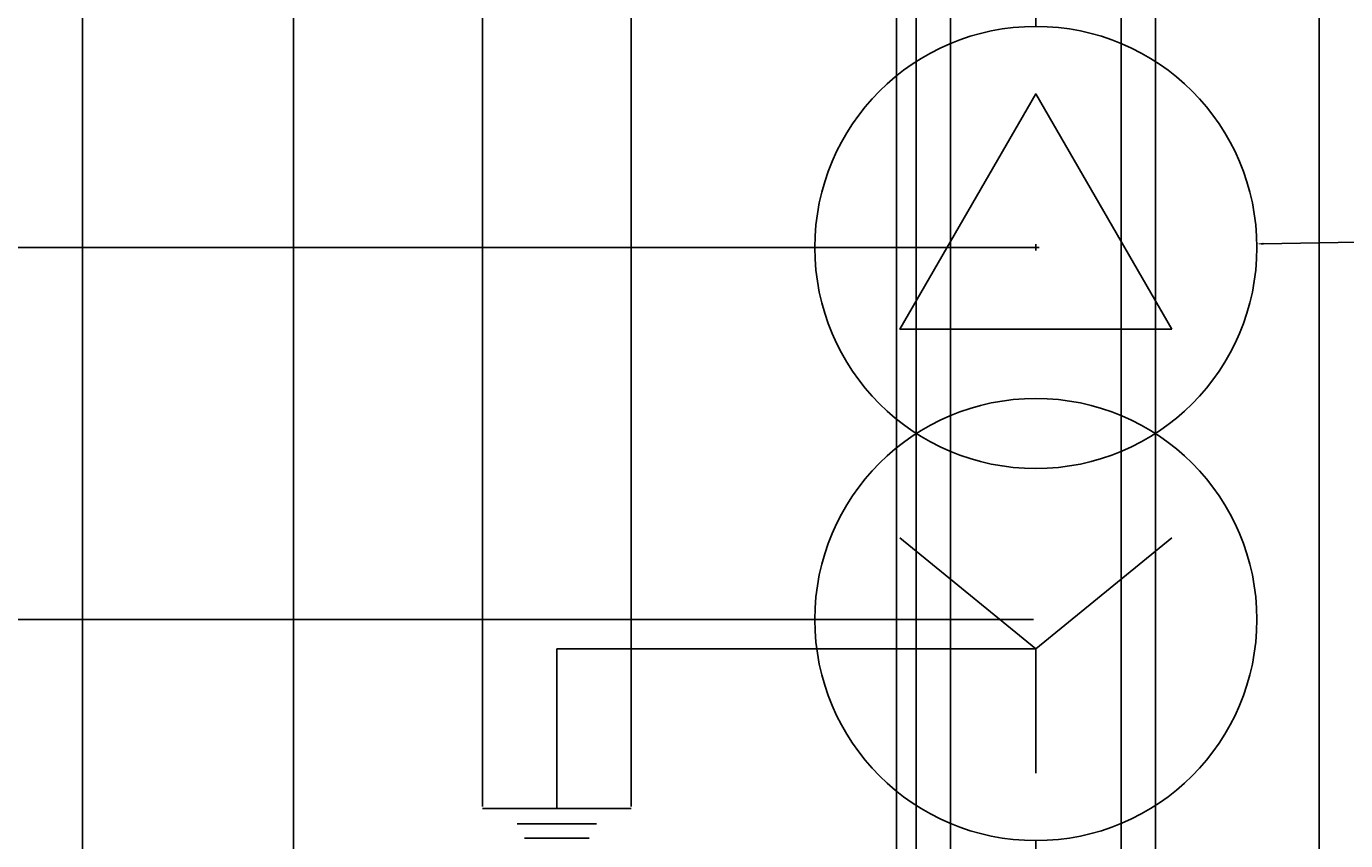
# Model space of a CAD drawing. Units: inches. Extents: x 412 to 584, y 208 to 437.
# Tile 17 of 28: x 471 to 508, y 315 to 338. Entities that reach past the tile are written whole.
import ezdxf

# ---------------------------------------------------------------- set-up
doc = ezdxf.new("R2010")
doc.units = ezdxf.units.IN
doc.header["$MEASUREMENT"] = 0
doc.layers.add('A-ANNO-DIMS', color=2, linetype='Continuous', lineweight=18)
doc.layers.add('E-POWR-EQPM', color=3, linetype='Continuous', lineweight=25)
doc.styles.get("Standard").update_dxf_attribs({"font": 'arial.ttf'})
doc.dimstyles.get("Standard").update_dxf_attribs({"dimtxt": 0.18, "dimasz": 0.18, "dimexe": 0.18, "dimexo": 0.0625, "dimgap": 0.09, "dimtad": 0, "dimtih": 1, "dimtoh": 1, "dimdec": 4, "dimzin": 0, "dimdsep": 46, "dimtxsty": 'Standard', "dimcen": 0.09, "dimadec": 0, "dimazin": 0, "dimtfac": 1, "dimtdec": 4, "dimtofl": 0, "dimtmove": 0, "dimatfit": 3, "dimfxl": 1, "dimtolj": 1, "dimtzin": 0, "dimarcsym": 0})

# ---------------------------------------------------------------- blocks, each defined once
blk = doc.blocks.new('*D17')
at = {"layer": 'A-ANNO-DIMS', "color": 0, "lineweight": -2, "transparency": 16777216}
for p, q in [((497.715, 426.185), (583.674, 426.185)), ((583.494, 426.005), (583.494, 323.031)), ((583.494, 219.693), (583.494, 322.667)), ((550.198, 219.513), (583.674, 219.513))]:
    blk.add_line(p, q, dxfattribs=at)
at = {"layer": 'A-ANNO-DIMS', "color": 0, "transparency": 16777216}
for points in [[(583.464, 426.005), (583.524, 426.005), (583.494, 426.185)], [(583.464, 219.693), (583.524, 219.693), (583.494, 219.513)]]:
    blk.add_solid(points, dxfattribs=at)
at = {"layer": 'Defpoints', "color": 0, "transparency": 16777216}
for p in [(497.652, 426.185), (550.135, 219.513), (583.494, 219.513)]:
    blk.add_point(p, dxfattribs=at)
at = {"layer": 'A-ANNO-DIMS', "color": 0, "transparency": 16777216, "insert": (583.494, 322.849), "char_height": 0.18, "attachment_point": 5}
blk.add_mtext('\\A1;206.67', dxfattribs=at)
blk = doc.blocks.new('*D24')
at = {"layer": 'A-ANNO-DIMS', "color": 0, "lineweight": -2, "transparency": 16777216}
for p, q in [((499.225, 349.373), (412.276, 349.373)), ((412.456, 349.193), (412.456, 340.743)), ((412.456, 331.93), (412.456, 340.38)), ((499.225, 331.75), (412.276, 331.75))]:
    blk.add_line(p, q, dxfattribs=at)
at = {"layer": 'A-ANNO-DIMS', "color": 0, "transparency": 16777216}
for points in [[(412.426, 349.193), (412.486, 349.193), (412.456, 349.373)], [(412.426, 331.93), (412.486, 331.93), (412.456, 331.75)]]:
    blk.add_solid(points, dxfattribs=at)
at = {"layer": 'Defpoints', "color": 0, "transparency": 16777216}
for p in [(499.288, 349.373), (412.456, 331.75), (499.288, 331.75)]:
    blk.add_point(p, dxfattribs=at)
at = {"layer": 'A-ANNO-DIMS', "color": 0, "transparency": 16777216, "insert": (412.456, 340.561), "char_height": 0.18, "attachment_point": 5}
blk.add_mtext('\\A1;17.624', dxfattribs=at)
blk = doc.blocks.new('*D25')
at = {"layer": 'A-ANNO-DIMS', "color": 0, "lineweight": -2, "transparency": 16777216}
for p, q in [((499.225, 331.75), (412.276, 331.75)), ((412.456, 331.57), (412.456, 326.704)), ((412.456, 321.474), (412.456, 326.34)), ((499.225, 321.294), (412.276, 321.294))]:
    blk.add_line(p, q, dxfattribs=at)
at = {"layer": 'A-ANNO-DIMS', "color": 0, "transparency": 16777216}
for points in [[(412.426, 331.57), (412.486, 331.57), (412.456, 331.75)], [(412.426, 321.474), (412.486, 321.474), (412.456, 321.294)]]:
    blk.add_solid(points, dxfattribs=at)
at = {"layer": 'Defpoints', "color": 0, "transparency": 16777216}
for p in [(499.288, 331.75), (412.456, 321.294), (499.288, 321.294)]:
    blk.add_point(p, dxfattribs=at)
at = {"layer": 'A-ANNO-DIMS', "color": 0, "transparency": 16777216, "insert": (412.456, 326.522), "char_height": 0.18, "attachment_point": 5}
blk.add_mtext('\\A1;10.456', dxfattribs=at)
blk = doc.blocks.new('*D26')
at = {"layer": 'A-ANNO-DIMS', "color": 0, "lineweight": -2, "transparency": 16777216}
for p, q in [((499.225, 321.294), (412.276, 321.294)), ((412.456, 321.114), (412.456, 315.518)), ((412.456, 309.557), (412.456, 315.154)), ((423.494, 309.377), (412.276, 309.377))]:
    blk.add_line(p, q, dxfattribs=at)
at = {"layer": 'A-ANNO-DIMS', "color": 0, "transparency": 16777216}
for points in [[(412.426, 321.114), (412.486, 321.114), (412.456, 321.294)], [(412.426, 309.557), (412.486, 309.557), (412.456, 309.377)]]:
    blk.add_solid(points, dxfattribs=at)
at = {"layer": 'Defpoints', "color": 0, "transparency": 16777216}
for p in [(499.288, 321.294), (412.456, 309.377), (423.556, 309.377)]:
    blk.add_point(p, dxfattribs=at)
at = {"layer": 'A-ANNO-DIMS', "color": 0, "transparency": 16777216, "insert": (412.456, 315.336), "char_height": 0.18, "attachment_point": 5}
blk.add_mtext('\\A1;11.917', dxfattribs=at)
blk = doc.blocks.new('*D28')
at = {"layer": 'A-ANNO-DIMS', "color": 0, "lineweight": -2, "transparency": 16777216}
for p, q in [((450.562, 256.635), (450.562, 437.465)), ((450.742, 437.285), (502.724, 437.285)), ((555.616, 437.285), (503.634, 437.285)), ((555.796, 256.635), (555.796, 437.465))]:
    blk.add_line(p, q, dxfattribs=at)
at = {"layer": 'A-ANNO-DIMS', "color": 0, "transparency": 16777216}
for points in [[(450.742, 437.315), (450.742, 437.255), (450.562, 437.285)], [(555.616, 437.315), (555.616, 437.255), (555.796, 437.285)]]:
    blk.add_solid(points, dxfattribs=at)
at = {"layer": 'Defpoints', "color": 0, "transparency": 16777216}
for p in [(555.796, 437.285), (450.562, 256.573), (555.796, 256.573)]:
    blk.add_point(p, dxfattribs=at)
at = {"layer": 'A-ANNO-DIMS', "color": 0, "transparency": 16777216, "insert": (503.179, 437.285), "char_height": 0.18, "attachment_point": 5}
blk.add_mtext('\\A1;105.23', dxfattribs=at)
blk = doc.blocks.new('*D29')
at = {"layer": 'A-ANNO-DIMS', "color": 0, "lineweight": -2, "transparency": 16777216}
for p, q in [((495.927, 378.924), (495.927, 208.233)), ((502.649, 378.924), (502.649, 208.233)), ((496.107, 208.413), (498.895, 208.413)), ((502.469, 208.413), (499.681, 208.413))]:
    blk.add_line(p, q, dxfattribs=at)
at = {"layer": 'A-ANNO-DIMS', "color": 0, "transparency": 16777216}
for points in [[(496.107, 208.443), (496.107, 208.383), (495.927, 208.413)], [(502.469, 208.443), (502.469, 208.383), (502.649, 208.413)]]:
    blk.add_solid(points, dxfattribs=at)
at = {"layer": 'Defpoints', "color": 0, "transparency": 16777216}
for p in [(495.927, 378.987), (502.649, 378.987), (502.649, 208.413)]:
    blk.add_point(p, dxfattribs=at)
at = {"layer": 'A-ANNO-DIMS', "color": 0, "transparency": 16777216, "insert": (499.288, 208.413), "char_height": 0.18, "attachment_point": 5}
blk.add_mtext('\\A1;6.722', dxfattribs=at)
blk = doc.blocks.new('*D31')
at = {"layer": 'A-ANNO-DIMS', "color": 0, "lineweight": -2, "transparency": 16777216}
for p, q in [((495.375, 405.385), (495.375, 208.233)), ((507.254, 405.385), (507.254, 208.233)), ((495.555, 208.413), (500.929, 208.413)), ((507.074, 208.413), (501.7, 208.413))]:
    blk.add_line(p, q, dxfattribs=at)
at = {"layer": 'A-ANNO-DIMS', "color": 0, "transparency": 16777216}
for points in [[(495.555, 208.443), (495.555, 208.383), (495.375, 208.413)], [(507.074, 208.443), (507.074, 208.383), (507.254, 208.413)]]:
    blk.add_solid(points, dxfattribs=at)
at = {"layer": 'Defpoints', "color": 0, "transparency": 16777216}
for p in [(495.375, 405.448), (507.254, 405.448), (507.254, 208.413)]:
    blk.add_point(p, dxfattribs=at)
at = {"layer": 'A-ANNO-DIMS', "color": 0, "transparency": 16777216, "insert": (501.314, 208.413), "char_height": 0.18, "attachment_point": 5}
blk.add_mtext('\\A1;11.88', dxfattribs=at)
blk = doc.blocks.new('*D33')
at = {"layer": 'A-ANNO-DIMS', "color": 0, "lineweight": -2, "transparency": 16777216}
for p, q in [((472.49, 363.226), (472.49, 208.233)), ((478.422, 363.226), (478.422, 208.233)), ((472.67, 208.413), (475.064, 208.413)), ((478.242, 208.413), (475.849, 208.413))]:
    blk.add_line(p, q, dxfattribs=at)
at = {"layer": 'A-ANNO-DIMS', "color": 0, "transparency": 16777216}
for points in [[(472.67, 208.443), (472.67, 208.383), (472.49, 208.413)], [(478.242, 208.443), (478.242, 208.383), (478.422, 208.413)]]:
    blk.add_solid(points, dxfattribs=at)
at = {"layer": 'Defpoints', "color": 0, "transparency": 16777216}
for p in [(472.49, 363.289), (478.422, 363.289), (478.422, 208.413)]:
    blk.add_point(p, dxfattribs=at)
at = {"layer": 'A-ANNO-DIMS', "color": 0, "transparency": 16777216, "insert": (475.456, 208.413), "char_height": 0.18, "attachment_point": 5}
blk.add_mtext('\\A1;5.932', dxfattribs=at)
blk = doc.blocks.new('*D39')
at = {"layer": 'A-ANNO-DIMS', "color": 0, "lineweight": -2, "transparency": 16777216}
for p, q in [((496.891, 346.914), (496.891, 208.233)), ((501.685, 346.914), (501.685, 208.233)), ((497.071, 208.413), (498.891, 208.413)), ((501.505, 208.413), (499.685, 208.413))]:
    blk.add_line(p, q, dxfattribs=at)
at = {"layer": 'A-ANNO-DIMS', "color": 0, "transparency": 16777216}
for points in [[(497.071, 208.443), (497.071, 208.383), (496.891, 208.413)], [(501.505, 208.443), (501.505, 208.383), (501.685, 208.413)]]:
    blk.add_solid(points, dxfattribs=at)
at = {"layer": 'Defpoints', "color": 0, "transparency": 16777216}
for p in [(496.891, 346.977), (501.685, 346.977), (501.685, 208.413)]:
    blk.add_point(p, dxfattribs=at)
at = {"layer": 'A-ANNO-DIMS', "color": 0, "transparency": 16777216, "insert": (499.288, 208.413), "char_height": 0.18, "attachment_point": 5}
blk.add_mtext('\\A1;4.794', dxfattribs=at)
blk = doc.blocks.new('*D41')
at = {"layer": 'A-ANNO-DIMS', "color": 0, "lineweight": -2, "transparency": 16777216}
for p, q in [((483.735, 316.045), (483.735, 437.465)), ((483.915, 437.285), (485.429, 437.285)), ((487.737, 437.285), (486.222, 437.285)), ((487.917, 316.045), (487.917, 437.465))]:
    blk.add_line(p, q, dxfattribs=at)
at = {"layer": 'A-ANNO-DIMS', "color": 0, "transparency": 16777216}
for points in [[(483.915, 437.315), (483.915, 437.255), (483.735, 437.285)], [(487.737, 437.315), (487.737, 437.255), (487.917, 437.285)]]:
    blk.add_solid(points, dxfattribs=at)
at = {"layer": 'Defpoints', "color": 0, "transparency": 16777216}
for p in [(487.917, 437.285), (483.735, 315.982), (487.917, 315.982)]:
    blk.add_point(p, dxfattribs=at)
at = {"layer": 'A-ANNO-DIMS', "color": 0, "transparency": 16777216, "insert": (485.826, 437.285), "char_height": 0.18, "attachment_point": 5}
blk.add_mtext('\\A1;4.182', dxfattribs=at)
blk = doc.blocks.new('*D42')
at = {"layer": 'A-ANNO-DIMS', "color": 0, "lineweight": -2, "transparency": 16777216}
for p, q in [((509.226, 331.91), (505.679, 331.853)), ((499.198, 331.75), (499.378, 331.75)), ((499.288, 331.66), (499.288, 331.84))]:
    blk.add_line(p, q, dxfattribs=at)
at = {"layer": 'A-ANNO-DIMS', "color": 0, "transparency": 16777216}
blk.add_solid([(505.679, 331.883), (505.68, 331.823), (505.499, 331.85)], dxfattribs=at)
at = {"layer": 'Defpoints', "color": 0, "transparency": 16777216}
for p in [(505.499, 331.85), (493.077, 331.649)]:
    blk.add_point(p, dxfattribs=at)
at = {"layer": 'A-ANNO-DIMS', "color": 0, "transparency": 16777216, "insert": (509.977, 331.91), "char_height": 0.18, "attachment_point": 5}
blk.add_mtext('\\A1;2X ∅12.424', dxfattribs=at)

msp = doc.modelspace()

# ---------------------------------------------------------------- linework, layer by layer
at = {"layer": 'E-POWR-EQPM'}
for p, q in [((499.2878, 349.3734), (499.2878, 337.9617)), ((495.4695, 323.5923), (499.2878, 320.4705)), ((499.2878, 320.4705), (503.1062, 323.5923)), ((499.2878, 320.4705), (485.8257, 320.4705)), ((485.8257, 320.4705), (485.8257, 315.9821)), ((499.2878, 320.4705), (499.2878, 316.9787)), ((485.8257, 315.9821), (483.7347, 315.9821)), ((485.8257, 315.9821), (487.9167, 315.9821)), ((485.8257, 315.5573), (484.7151, 315.5573)), ((485.8257, 315.5573), (486.9363, 315.5573)), ((484.92, 315.1475), (486.7314, 315.1475)), ((499.2878, 315.082), (499.2878, 303.6727))]:
    msp.add_line(p, q, dxfattribs=at)
msp.add_lwpolyline([(503.1062, 329.4514), (499.2878, 336.065), (495.4695, 329.4514)], close=True, dxfattribs=at)
for centre in [(499.2878, 331.7496), (499.2878, 321.2941)]:
    msp.add_circle(centre, 6.2121, dxfattribs=at)

# ---------------------------------------------------------------- dimensions: what is measured, and where the dimension line sits
at = {"layer": 'A-ANNO-DIMS'}
for base, p1, p2, override, picture, middle in [((555.7959, 437.2847), (450.562, 256.5729), (555.7959, 256.5729), {"dimdec": 2, "dimlfac": 1, "dimrnd": 0, "dimzin": 0, "dimdsep": 46, "dimlunit": 2}, '*D28', (503.1789, 437.2847)), ((487.9167, 437.2847), (483.7347, 315.9821), (487.9167, 315.9821), {"dimdec": 3, "dimlfac": 1, "dimrnd": 0, "dimzin": 0, "dimdsep": 46, "dimlunit": 2}, '*D41', (485.8257, 437.2847)), ((507.2538, 208.4133), (495.3746, 405.448), (507.2538, 405.448), {"dimdec": 2, "dimlfac": 1, "dimrnd": 0, "dimzin": 0, "dimdsep": 46, "dimlunit": 2}, '*D31', (501.3142, 208.4133)), ((502.6489, 208.4133), (495.9268, 378.9867), (502.6489, 378.9867), {"dimdec": 3, "dimlfac": 1, "dimrnd": 0, "dimzin": 0, "dimdsep": 46, "dimlunit": 2}, '*D29', (499.2878, 208.4133)), ((478.4225, 208.4133), (472.4903, 363.2888), (478.4225, 363.2888), {"dimdec": 3, "dimlfac": 1, "dimrnd": 0, "dimzin": 0, "dimdsep": 46, "dimlunit": 2}, '*D33', (475.4564, 208.4133)), ((501.6846, 208.4133), (496.891, 346.9765), (501.6846, 346.9765), {"dimdec": 3, "dimlfac": 1, "dimrnd": 0, "dimzin": 0, "dimdsep": 46, "dimlunit": 2}, '*D39', (499.2878, 208.4133))]:
    dim = msp.add_linear_dim(base=base, p1=p1, p2=p2, dimstyle='Standard', override=override, dxfattribs=at)
    dim.commit()
    dim.dimension.update_dxf_attribs({"geometry": picture, "text_midpoint": middle})
for base, p1, p2, override, picture, middle in [((583.4937, 219.5133), (497.6523, 426.1847), (550.1351, 219.5133), {"dimdec": 2, "dimlfac": 1, "dimrnd": 0, "dimzin": 0, "dimdsep": 46, "dimlunit": 2}, '*D17', (583.4937, 322.849)), ((412.4562, 331.7496), (499.2878, 349.3734), (499.2878, 331.7496), {"dimdec": 3, "dimlfac": 1, "dimrnd": 0, "dimzin": 0, "dimdsep": 46, "dimlunit": 2}, '*D24', (412.4562, 340.5615)), ((412.45622, 321.29408), (499.28783, 331.74962), (499.28783, 321.29408), {"dimdec": 3, "dimlfac": 1, "dimrnd": 0, "dimzin": 0, "dimdsep": 46, "dimlunit": 2}, '*D25', (412.45622, 326.52185)), ((412.4562, 309.3773), (499.2878, 321.2941), (423.5562, 309.3773), {"dimdec": 3, "dimlfac": 1, "dimrnd": 0, "dimzin": 0, "dimdsep": 46, "dimlunit": 2}, '*D26', (412.4562, 315.3357))]:
    dim = msp.add_linear_dim(base=base, p1=p1, p2=p2, angle=90, dimstyle='Standard', override=override, dxfattribs=at)
    dim.commit()
    dim.dimension.update_dxf_attribs({"geometry": picture, "text_midpoint": middle})
dim = msp.add_diameter_dim_2p(p1=(493.0765, 331.6491), p2=(505.4991, 331.8501), text='2X <>', dimstyle='Standard', override={"dimdec": 3, "dimlfac": 1, "dimrnd": 0, "dimzin": 0, "dimdsep": 46, "dimlunit": 2}, dxfattribs=at)
dim.commit()
dim.dimension.update_dxf_attribs({"geometry": '*D42', "text_midpoint": (509.2259, 331.9105), "dimtype": 163})

doc.saveas('drawing.dxf')
